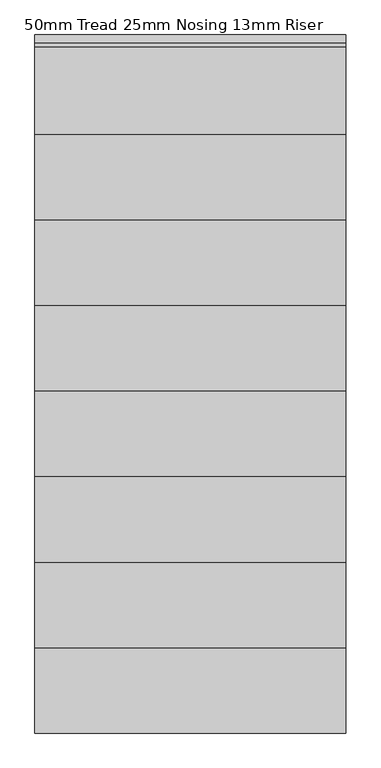
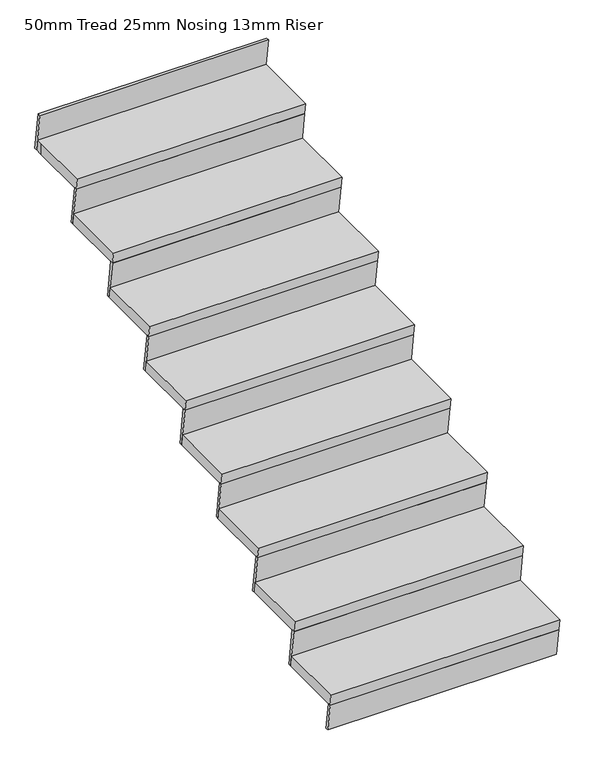
"""IFC4 building model written with IfcOpenShell, lengths in millimetres: stair flight geometry, 50mm Tread 25mm Nosing 13mm Riser."""

from ifc_helpers import new_model, si_unit, origin, place, context, project, spatial, faceted_brep, source, transform, mapped, element, save


def stair_flight_50mm_tread_25mm_nosing_13mm_riser_f1e983ca(model_context):
    return source(origin(), model_context, "Body", "Brep", [
        faceted_brep([(-11022.1547869, 1127.4280728, 173.9130435), (-11022.1547869, 1134.6155728, 123.9130435), (-12022.1805681, 1134.6155728, 123.9130435), (-12022.1805681, 1127.4280728, 173.9130435), (-12022.1805681, 827.4280728, 173.9130435), (-11022.1547869, 827.4280728, 173.9130435), (-11022.1547869, 834.6155728, 123.9130435), (-12022.1805681, 834.6155728, 123.9130435)], [[[0, 1, 2, 3]], [[3, 4, 5, 0]], [[2, 1, 6, 7]], [[4, 3, 2, 7]], [[0, 5, 6, 1]], [[5, 4, 7, 6]]]),
        faceted_brep([(-11022.1547869, 834.6155728, 123.9130435), (-11022.1547869, 852.4280728, 0.0), (-11022.1547869, 865.0565628, 0.0), (-11022.1547869, 847.2440628, 123.9130435), (-12022.1805681, 834.6155728, 123.9130435), (-12022.1805681, 847.2440628, 123.9130435), (-12022.1805681, 865.0565628, 0.0), (-12022.1805681, 852.4280728, 0.0)], [[[0, 1, 2, 3]], [[4, 5, 6, 7]], [[1, 0, 4, 7]], [[2, 1, 7, 6]], [[3, 2, 6, 5]], [[0, 3, 5, 4]]]),
        faceted_brep([(-11022.1547869, 1109.6155728, 297.826087), (-11022.1547869, 1134.6155728, 123.9130435), (-11022.1547869, 1147.2440628, 123.9130435), (-11022.1547869, 1122.2440628, 297.826087), (-12022.1805681, 1109.6155728, 297.826087), (-12022.1805681, 1122.2440628, 297.826087), (-12022.1805681, 1147.2440628, 123.9130435), (-12022.1805681, 1134.6155728, 123.9130435)], [[[0, 1, 2, 3]], [[4, 5, 6, 7]], [[1, 0, 4, 7]], [[2, 1, 7, 6]], [[3, 2, 6, 5]], [[0, 3, 5, 4]]]),
        faceted_brep([(-12022.1805681, 1402.4280728, 347.826087), (-12022.1805681, 1102.4280728, 347.826087), (-11022.1547869, 1102.4280728, 347.826087), (-11022.1547869, 1402.4280728, 347.826087), (-12022.1805681, 1409.6155728, 297.826087), (-11022.1547869, 1409.6155728, 297.826087), (-11022.1547869, 1109.6155728, 297.826087), (-12022.1805681, 1109.6155728, 297.826087)], [[[0, 1, 2, 3]], [[4, 5, 6, 7]], [[1, 0, 4, 7]], [[3, 2, 6, 5]], [[3, 5, 4, 0]], [[2, 1, 7, 6]]]),
        faceted_brep([(-11022.1547869, 1384.6155728, 471.7391304), (-11022.1547869, 1409.6155728, 297.826087), (-11022.1547869, 1422.2440628, 297.826087), (-11022.1547869, 1397.2440628, 471.7391304), (-12022.1805681, 1384.6155728, 471.7391304), (-12022.1805681, 1397.2440628, 471.7391304), (-12022.1805681, 1422.2440628, 297.826087), (-12022.1805681, 1409.6155728, 297.826087)], [[[0, 1, 2, 3]], [[4, 5, 6, 7]], [[1, 0, 4, 7]], [[2, 1, 7, 6]], [[3, 2, 6, 5]], [[0, 3, 5, 4]]]),
        faceted_brep([(-12022.1805681, 1677.4280728, 521.7391304), (-12022.1805681, 1377.4280728, 521.7391304), (-11022.1547869, 1377.4280728, 521.7391304), (-11022.1547869, 1677.4280728, 521.7391304), (-12022.1805681, 1684.6155728, 471.7391304), (-11022.1547869, 1684.6155728, 471.7391304), (-11022.1547869, 1384.6155728, 471.7391304), (-12022.1805681, 1384.6155728, 471.7391304)], [[[0, 1, 2, 3]], [[4, 5, 6, 7]], [[1, 0, 4, 7]], [[3, 2, 6, 5]], [[3, 5, 4, 0]], [[2, 1, 7, 6]]]),
        faceted_brep([(-11022.1547869, 1659.6155728, 645.6521739), (-11022.1547869, 1684.6155728, 471.7391304), (-11022.1547869, 1697.2440628, 471.7391304), (-11022.1547869, 1672.2440628, 645.6521739), (-12022.1805681, 1659.6155728, 645.6521739), (-12022.1805681, 1672.2440628, 645.6521739), (-12022.1805681, 1697.2440628, 471.7391304), (-12022.1805681, 1684.6155728, 471.7391304)], [[[0, 1, 2, 3]], [[4, 5, 6, 7]], [[1, 0, 4, 7]], [[2, 1, 7, 6]], [[3, 2, 6, 5]], [[0, 3, 5, 4]]]),
        faceted_brep([(-12022.1805681, 1952.4280728, 695.6521739), (-12022.1805681, 1652.4280728, 695.6521739), (-11022.1547869, 1652.4280728, 695.6521739), (-11022.1547869, 1952.4280728, 695.6521739), (-12022.1805681, 1959.6155728, 645.6521739), (-11022.1547869, 1959.6155728, 645.6521739), (-11022.1547869, 1659.6155728, 645.6521739), (-12022.1805681, 1659.6155728, 645.6521739)], [[[0, 1, 2, 3]], [[4, 5, 6, 7]], [[1, 0, 4, 7]], [[3, 2, 6, 5]], [[3, 5, 4, 0]], [[2, 1, 7, 6]]]),
        faceted_brep([(-11022.1547869, 1934.6155728, 819.5652174), (-11022.1547869, 1959.6155728, 645.6521739), (-11022.1547869, 1972.2440628, 645.6521739), (-11022.1547869, 1947.2440628, 819.5652174), (-12022.1805681, 1934.6155728, 819.5652174), (-12022.1805681, 1947.2440628, 819.5652174), (-12022.1805681, 1972.2440628, 645.6521739), (-12022.1805681, 1959.6155728, 645.6521739)], [[[0, 1, 2, 3]], [[4, 5, 6, 7]], [[1, 0, 4, 7]], [[2, 1, 7, 6]], [[3, 2, 6, 5]], [[0, 3, 5, 4]]]),
        faceted_brep([(-12022.1805681, 2227.4280728, 869.5652174), (-12022.1805681, 1927.4280728, 869.5652174), (-11022.1547869, 1927.4280728, 869.5652174), (-11022.1547869, 2227.4280728, 869.5652174), (-12022.1805681, 2234.6155728, 819.5652174), (-11022.1547869, 2234.6155728, 819.5652174), (-11022.1547869, 1934.6155728, 819.5652174), (-12022.1805681, 1934.6155728, 819.5652174)], [[[0, 1, 2, 3]], [[4, 5, 6, 7]], [[1, 0, 4, 7]], [[3, 2, 6, 5]], [[3, 5, 4, 0]], [[2, 1, 7, 6]]]),
        faceted_brep([(-11022.1547869, 2209.6155728, 993.4782609), (-11022.1547869, 2234.6155728, 819.5652174), (-11022.1547869, 2247.2440628, 819.5652174), (-11022.1547869, 2222.2440628, 993.4782609), (-12022.1805681, 2209.6155728, 993.4782609), (-12022.1805681, 2222.2440628, 993.4782609), (-12022.1805681, 2247.2440628, 819.5652174), (-12022.1805681, 2234.6155728, 819.5652174)], [[[0, 1, 2, 3]], [[4, 5, 6, 7]], [[1, 0, 4, 7]], [[2, 1, 7, 6]], [[3, 2, 6, 5]], [[0, 3, 5, 4]]]),
        faceted_brep([(-12022.1805681, 2502.4280728, 1043.4782609), (-12022.1805681, 2202.4280728, 1043.4782609), (-11022.1547869, 2202.4280728, 1043.4782609), (-11022.1547869, 2502.4280728, 1043.4782609), (-12022.1805681, 2509.6155728, 993.4782609), (-11022.1547869, 2509.6155728, 993.4782609), (-11022.1547869, 2209.6155728, 993.4782609), (-12022.1805681, 2209.6155728, 993.4782609)], [[[0, 1, 2, 3]], [[4, 5, 6, 7]], [[1, 0, 4, 7]], [[3, 2, 6, 5]], [[3, 5, 4, 0]], [[2, 1, 7, 6]]]),
        faceted_brep([(-11022.1547869, 2484.6155728, 1167.3913043), (-11022.1547869, 2509.6155728, 993.4782609), (-11022.1547869, 2522.2440628, 993.4782609), (-11022.1547869, 2497.2440628, 1167.3913043), (-12022.1805681, 2484.6155728, 1167.3913043), (-12022.1805681, 2497.2440628, 1167.3913043), (-12022.1805681, 2522.2440628, 993.4782609), (-12022.1805681, 2509.6155728, 993.4782609)], [[[0, 1, 2, 3]], [[4, 5, 6, 7]], [[1, 0, 4, 7]], [[2, 1, 7, 6]], [[3, 2, 6, 5]], [[0, 3, 5, 4]]]),
        faceted_brep([(-12022.1805681, 2777.4280728, 1217.3913043), (-12022.1805681, 2477.4280728, 1217.3913043), (-11022.1547869, 2477.4280728, 1217.3913043), (-11022.1547869, 2777.4280728, 1217.3913043), (-12022.1805681, 2784.6155728, 1167.3913043), (-11022.1547869, 2784.6155728, 1167.3913043), (-11022.1547869, 2484.6155728, 1167.3913043), (-12022.1805681, 2484.6155728, 1167.3913043)], [[[0, 1, 2, 3]], [[4, 5, 6, 7]], [[1, 0, 4, 7]], [[3, 2, 6, 5]], [[3, 5, 4, 0]], [[2, 1, 7, 6]]]),
        faceted_brep([(-11022.1547869, 3034.6155728, 1515.2173913), (-11022.1547869, 3059.6155728, 1341.3043478), (-11022.1547869, 3072.2440628, 1341.3043478), (-11022.1547869, 3047.2440628, 1515.2173913), (-12022.1805681, 3034.6155728, 1515.2173913), (-12022.1805681, 3047.2440628, 1515.2173913), (-12022.1805681, 3072.2440628, 1341.3043478), (-12022.1805681, 3059.6155728, 1341.3043478)], [[[0, 1, 2, 3]], [[4, 5, 6, 7]], [[1, 0, 4, 7]], [[2, 1, 7, 6]], [[3, 2, 6, 5]], [[0, 3, 5, 4]]]),
        faceted_brep([(-11022.1547869, 2759.6155728, 1341.3043478), (-11022.1547869, 2784.6155728, 1167.3913043), (-11022.1547869, 2797.2440628, 1167.3913043), (-11022.1547869, 2772.2440628, 1341.3043478), (-12022.1805681, 2759.6155728, 1341.3043478), (-12022.1805681, 2772.2440628, 1341.3043478), (-12022.1805681, 2797.2440628, 1167.3913043), (-12022.1805681, 2784.6155728, 1167.3913043)], [[[0, 1, 2, 3]], [[4, 5, 6, 7]], [[1, 0, 4, 7]], [[2, 1, 7, 6]], [[3, 2, 6, 5]], [[0, 3, 5, 4]]]),
        faceted_brep([(-12022.1805681, 3052.4280728, 1391.3043478), (-12022.1805681, 3027.4280728, 1391.3043478), (-12022.1805681, 2752.4280728, 1391.3043478), (-11022.1547869, 2752.4280728, 1391.3043478), (-11022.1547869, 3052.4280728, 1391.3043478), (-12022.1805681, 3059.6155728, 1341.3043478), (-11022.1547869, 3059.6155728, 1341.3043478), (-11022.1547869, 2759.6155728, 1341.3043478), (-12022.1805681, 2759.6155728, 1341.3043478), (-12022.1805681, 3027.4280728, 1341.3043478)], [[[0, 1, 2, 3, 4]], [[5, 6, 7, 8, 9]], [[1, 0, 5, 9]], [[2, 1, 9, 8]], [[4, 3, 7, 6]], [[4, 6, 5, 0]], [[3, 2, 8, 7]]]),
    ])


if __name__ == "__main__":
    model = new_model("IFC4")
    model_context = context("Model", 3, world=origin())
    ifc_project = project(units=[si_unit("LENGTHUNIT", "METRE", prefix="MILLI")], contexts=[model_context])
    site = spatial("IfcSite", under=ifc_project)
    building = spatial("IfcBuilding", under=site)
    placement = place(None, origin())
    stair_flight_50mm_tread_25mm_nosing_13mm_riser_shape = stair_flight_50mm_tread_25mm_nosing_13mm_riser_f1e983ca(model_context)
    element("IfcStairFlight", 1, ObjectType="50mm Tread 25mm Nosing 13mm Riser", at=placement, inside=building, context=model_context, shape_type="MappedRepresentation", body=[
        mapped(stair_flight_50mm_tread_25mm_nosing_13mm_riser_shape, transform((0.0, 0.0, 0.0), x_axis=(1.0, 0.0, 0.0), y_axis=(0.0, 1.0, 0.0), z_axis=(0.0, 0.0, 1.0))),
    ])
    save(model, "model.ifc")
